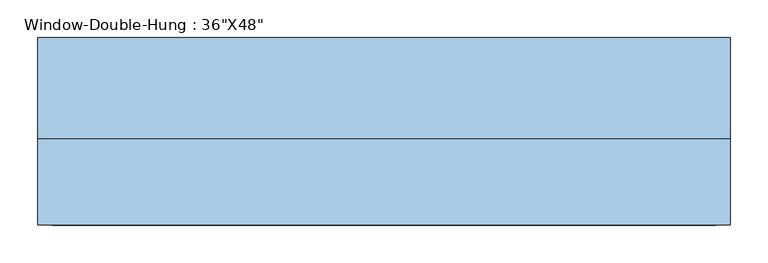
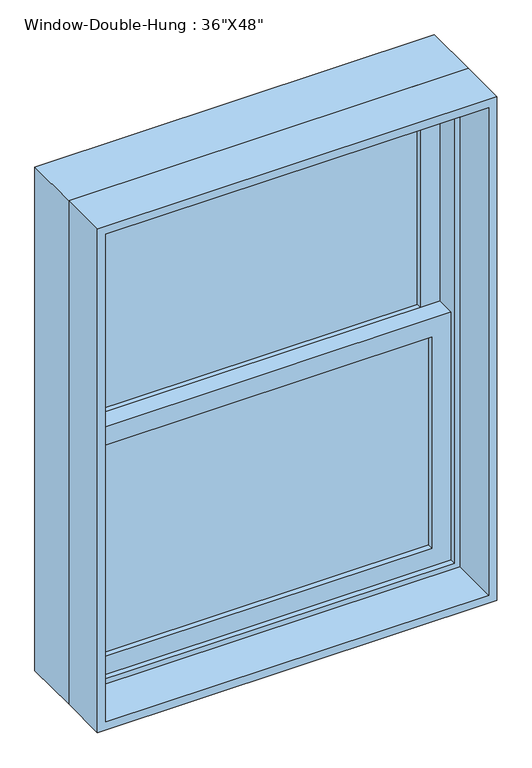
"""IFC4 building model written with IfcOpenShell, lengths in millimetres: window geometry."""

from ifc_helpers import new_model, si_unit, frame, origin, place, context, project, spatial, polyline, outline, extrude, source, transform, mapped, element, save


def window_559c395e(model_context):
    return source(origin(), model_context, "Body", "SweptSolid", [
        extrude(outline(polyline([(381.0, 44.45), (381.0, 38.1), (-381.0, 38.1), (-381.0, 44.45), (381.0, 44.45)])), frame((0.0, 0.0, 990.6), z_axis=(0.0, 0.0, 1.0), x_axis=(1.0, 0.0, 0.0)), (0.0, 0.0, 1.0), 511.175),
        extrude(outline(polyline([(-381.0, 31.75), (381.0, 31.75), (381.0, 25.4), (-381.0, 25.4), (-381.0, 31.75)])), frame((0.0, 0.0, 990.6), z_axis=(0.0, 0.0, 1.0), x_axis=(1.0, 0.0, 0.0)), (0.0, 0.0, 1.0), 511.175),
        extrude(outline(polyline([(381.0, 88.9), (381.0, 82.55), (-381.0, 82.55), (-381.0, 88.9), (381.0, 88.9)])), frame((0.0, 0.0, 1546.225), z_axis=(0.0, 0.0, 1.0), x_axis=(1.0, 0.0, 0.0)), (0.0, 0.0, 1.0), 511.175),
        extrude(outline(polyline([(-381.0, 76.2), (381.0, 76.2), (381.0, 69.85), (-381.0, 69.85), (-381.0, 76.2)])), frame((0.0, 0.0, 1546.225), z_axis=(0.0, 0.0, 1.0), x_axis=(1.0, 0.0, 0.0)), (0.0, 0.0, 1.0), 511.175),
        extrude(outline(polyline([(1546.225, -425.45), (946.15, -425.45), (946.15, 425.45), (1546.225, 425.45), (1546.225, -425.45)]), holes=[polyline([(1501.775, 381.0), (990.6, 381.0), (990.6, -381.0), (1501.775, -381.0), (1501.775, 381.0)])]), frame((0.0, 12.7, 0.0), z_axis=(0.0, 1.0, 0.0), x_axis=(0.0, 0.0, 1.0)), (0.0, 0.0, 1.0), 44.45),
        extrude(outline(polyline([(2101.85, -425.45), (1501.775, -425.45), (1501.775, 425.45), (2101.85, 425.45), (2101.85, -425.45)]), holes=[polyline([(2057.4, 381.0), (1546.225, 381.0), (1546.225, -381.0), (2057.4, -381.0), (2057.4, 381.0)])]), frame((0.0, 57.15, 0.0), z_axis=(0.0, 1.0, 0.0), x_axis=(0.0, 0.0, 1.0)), (0.0, 0.0, 1.0), 44.45),
        extrude(outline(polyline([(2133.6, -457.2), (914.4, -457.2), (914.4, 457.2), (2133.6, 457.2), (2133.6, -457.2)]), holes=[polyline([(2101.85, 425.45), (946.15, 425.45), (946.15, -425.45), (2101.85, -425.45), (2101.85, 425.45)])]), frame((0.0, 0.0, 0.0), z_axis=(0.0, 1.0, 0.0), x_axis=(0.0, 0.0, 1.0)), (0.0, 0.0, 1.0), 133.35),
        extrude(outline(polyline([(2133.6, 457.2), (2133.6, -457.2), (914.4, -457.2), (914.4, 457.2), (2133.6, 457.2)]), holes=[polyline([(2114.55, 438.15), (933.45, 438.15), (933.45, -438.15), (2114.55, -438.15), (2114.55, 438.15)])]), frame((0.0, -114.3, 0.0), z_axis=(0.0, 1.0, 0.0), x_axis=(0.0, 0.0, 1.0)), (0.0, 0.0, 1.0), 114.3),
    ])


if __name__ == "__main__":
    model = new_model("IFC4")
    model_context = context("Model", 3, world=origin())
    ifc_project = project(units=[si_unit("LENGTHUNIT", "METRE", prefix="MILLI")], contexts=[model_context])
    site = spatial("IfcSite", under=ifc_project)
    building = spatial("IfcBuilding", under=site)
    placement = place(None, origin())
    window_shape = window_559c395e(model_context)
    element("IfcWindow", 1, ObjectType="Window-Double-Hung : 36\"X48\"", at=placement, inside=building, context=model_context, shape_type="MappedRepresentation", body=[
        mapped(window_shape, transform((0.0, 0.0, 0.0), x_axis=(1.0, 0.0, 0.0), y_axis=(0.0, 1.0, 0.0), z_axis=(0.0, 0.0, 1.0))),
    ])
    save(model, "model.ifc")

# Revit data of these elements
# Type "Window-Double-Hung : 36\"X48\""
#   Type Mark = "21"
#   Fire Rating = "0.5h"
#   Construction Type Id = "DG-DR"
#   Assembly Code = "B2020100"
#   Analytic Construction = "Double glazing - domestic"
#   Wall Thickness [instance default] = 0' - 6"
#   Window Inset [instance default] = 0' - 0"
#   Visual Light Transmittance = 0.81
#   Thermal Resistance (R) = 1.8146 (h·ft²·°F)/BTU
#   Solar Heat Gain Coefficient = 0.76
#   Muntin Width = 2' - 6"
#   Muntin Height = 1' - 8 1/8"
#   Interior Wall Closure [instance default] = 0' - 1 1/2"
#   Rough Width = 3' - 0 1/2"
#   Rough Height = 4' - 0 1/2"
#   Frame Extension [instance default] = 0' - 1 1/4"
#   Exterior Wall Closure [instance default] = 0' - 0 1/2"
#   Extension Jamb [instance default] = 0' - 1 1/2"
#   Heat Transfer Coefficient (U) = 0.5511 BTU/(h·ft²·°F)
#   Height = 4' - 0"
#   Width = 3' - 0"
#   Top Muntin Visibility = yes
#   Indicator Visibility [instance default] = yes
#   Extension Jamb Visibility [instance default] = yes
#   Interior Trim Visibility [instance default] = yes
#   Exterior Trim Visibility [instance default] = yes
#   Define Thermal Properties by = 1
#   Bottom Muntin Visibility = yes
#   Muntin Pattern = Muntin Pattern_2x2 : Muntin Pattern_2x2
#   Interior Trim Material = Wood - Stained
#   Interior Trim = Trim-Window-Interior-Flat : Picture Frame
#   Exterior Trim Material = Clad - White
#   Exterior Trim = Trim-Window-Exterior-Flat : with Sill
#   Glass Panel Material = Glass
#   Exterior Frame Material = Clad - White
#   Interior Frame Material = Wood - Stained
#   Wall Closure = (empty or 0)
# Element 1 (IfcWindow, "Window-Double-Hung : 36\"X48\"")
#   Wall Thickness = 0' - 9"
#   Extension Jamb = 0' - 4 1/2"
#   Materials on its faces: "Wood - Stained", "Glass", "Clad - White"
# Materials
#   "Wood - Stained": class "Wood", colour RGB 224 178 126, transparency 0, Cost = 0
#   "Clad - White": class "Wood", colour RGB 242 242 238, transparency 0, Cost = 0
#   "Glass": class "Glass", colour RGB 0 128 192, transparency 0.75, Description = "Soda Lime Glass", Cost = 0
